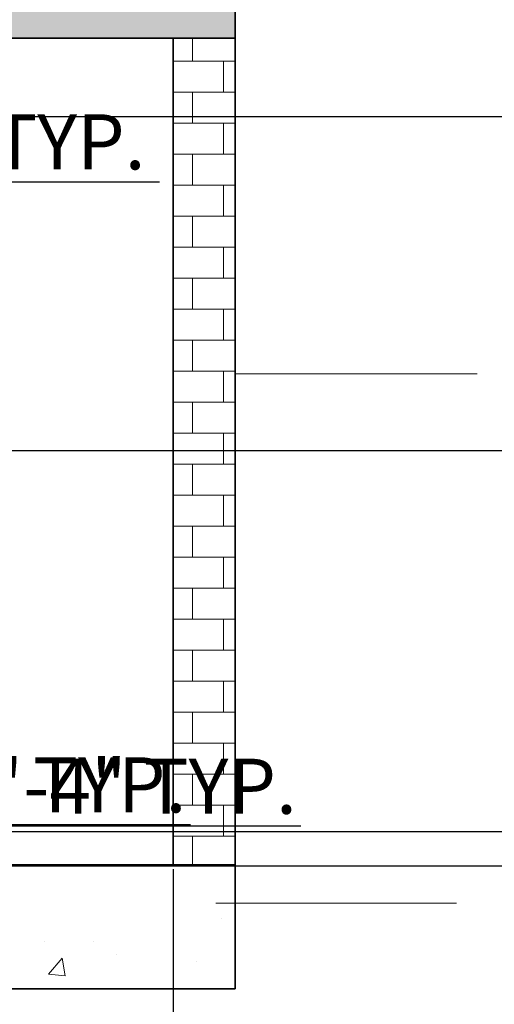
# Model space of a CAD drawing. Units: inches. Extents: x 2257 to 3678, y 834 to 1975.
# Tile 14 of 16: x 3471 to 3540, y 1677 to 1820. Entities that reach past the tile are written whole.
import ezdxf

# ---------------------------------------------------------------- set-up
doc = ezdxf.new("R2010")
doc.units = ezdxf.units.IN
for name, color, linetype, lineweight in [('A-ANNO-DIMS', 2, 'Continuous', 18), ('A-ANNO-TEXT', 7, 'Continuous', 18), ('A-SECT', 7, 'Continuous', 35), ('A-SECT-BRCK-PATT', 252, 'Continuous', 13), ('A-SECT-CONC-PATT', 252, 'Continuous', 13)]:
    doc.layers.add(name, color=color, linetype=linetype, lineweight=lineweight)
doc.styles.get("Standard").update_dxf_attribs({"font": 'arial.ttf'})
doc.dimstyles.new('ISO-25', dxfattribs={"dimtxt": 8, "dimasz": 2.5, "dimexe": 1.25, "dimexo": 0.625, "dimtad": 1, "dimdec": 0, "dimlunit": 3, "dimtxsty": 'Standard', "dimcen": 2.5, "dimadec": 0, "dimazin": 0, "dimtfac": 1, "dimtdec": 0, "dimtmove": 0, "dimatfit": 3, "dimfxl": 1, "dimarcsym": 0})

# ---------------------------------------------------------------- blocks, each defined once
blk = doc.blocks.new('*D84')
at = {"layer": 'A-ANNO-DIMS', "color": 0, "lineweight": -2, "transparency": 16777216}
for p, q in [((3377.06, 1793.76), (3377.06, 1797.23)), ((3396.05, 1793.76), (3396.05, 1797.23)), ((3379.56, 1795.98), (3393.55, 1795.98)), ((3396.05, 1795.98), (3491.69, 1795.98))]:
    blk.add_line(p, q, dxfattribs=at)
at = {"layer": 'A-ANNO-DIMS', "color": 0, "transparency": 16777216}
for points in [[(3379.56, 1796.4), (3379.56, 1795.56), (3377.06, 1795.98)], [(3393.55, 1796.4), (3393.55, 1795.56), (3396.05, 1795.98)]]:
    blk.add_solid(points, dxfattribs=at)
at = {"layer": 'Defpoints', "color": 0, "transparency": 16777216}
for p in [(3396.05, 1795.98), (3377.06, 1793.13), (3396.05, 1793.13)]:
    blk.add_point(p, dxfattribs=at)
at = {"layer": 'A-ANNO-DIMS', "color": 0, "transparency": 16777216, "insert": (3445.12, 1800.74), "char_height": 8, "attachment_point": 5}
blk.add_mtext('LINENS 1\'-7" TYP.', dxfattribs=at)
blk = doc.blocks.new('*D90')
at = {"layer": 'A-ANNO-DIMS', "color": 0, "lineweight": -2, "transparency": 16777216}
for p, q in [((3463.51, 1750.62), (3463.51, 1883.51)), ((3457.86, 1750.62), (3464.76, 1750.62)), ((3463.51, 1711.27), (3463.51, 1748.12)), ((3457.86, 1708.77), (3464.76, 1708.77))]:
    blk.add_line(p, q, dxfattribs=at)
at = {"layer": 'A-ANNO-DIMS', "color": 0, "transparency": 16777216}
for points in [[(3463.09, 1748.12), (3463.92, 1748.12), (3463.51, 1750.62)], [(3463.09, 1711.27), (3463.92, 1711.27), (3463.51, 1708.77)]]:
    blk.add_solid(points, dxfattribs=at)
at = {"layer": 'Defpoints', "color": 0, "transparency": 16777216}
for p in [(3457.23, 1750.62), (3463.51, 1750.62), (3457.23, 1708.77)]:
    blk.add_point(p, dxfattribs=at)
at = {"layer": 'A-ANNO-DIMS', "color": 0, "transparency": 16777216, "insert": (3458.74, 1818.32), "char_height": 8, "attachment_point": 5, "rotation": 90}
blk.add_mtext('LONG JACKET 3\'-6" TYP.', dxfattribs=at)
blk = doc.blocks.new('*D91')
at = {"layer": 'A-ANNO-DIMS', "color": 0, "lineweight": -2, "transparency": 16777216}
for p, q in [((3453, 1708.14), (3453, 1701.24)), ((3457.23, 1708.14), (3457.23, 1701.24)), ((3450.5, 1702.49), (3448, 1702.49)), ((3453, 1702.49), (3457.23, 1702.49)), ((3459.73, 1702.49), (3512.24, 1702.49))]:
    blk.add_line(p, q, dxfattribs=at)
at = {"layer": 'A-ANNO-DIMS', "color": 0, "transparency": 16777216}
for points in [[(3450.5, 1702.91), (3450.5, 1702.08), (3453, 1702.49)], [(3459.73, 1702.91), (3459.73, 1702.08), (3457.23, 1702.49)]]:
    blk.add_solid(points, dxfattribs=at)
at = {"layer": 'Defpoints', "color": 0, "transparency": 16777216}
for p in [(3453, 1708.77), (3457.23, 1708.77), (3457.23, 1702.49)]:
    blk.add_point(p, dxfattribs=at)
at = {"layer": 'A-ANNO-DIMS', "color": 0, "transparency": 16777216, "insert": (3487.24, 1707.2), "char_height": 8, "attachment_point": 5}
blk.add_mtext('0\'-4" TYP.', dxfattribs=at)
blk = doc.blocks.new('*D93')
at = {"layer": 'A-ANNO-DIMS', "color": 0, "lineweight": -2, "transparency": 16777216}
for p, q in [((3435.17, 1708.31), (3435.17, 1701.44)), ((3441.18, 1708.31), (3441.18, 1701.44)), ((3432.67, 1702.69), (3430.17, 1702.69)), ((3435.17, 1702.69), (3441.18, 1702.69)), ((3443.68, 1702.69), (3496.2, 1702.69))]:
    blk.add_line(p, q, dxfattribs=at)
at = {"layer": 'A-ANNO-DIMS', "color": 0, "transparency": 16777216}
for points in [[(3432.67, 1703.11), (3432.67, 1702.27), (3435.17, 1702.69)], [(3443.68, 1703.11), (3443.68, 1702.27), (3441.18, 1702.69)]]:
    blk.add_solid(points, dxfattribs=at)
at = {"layer": 'Defpoints', "color": 0, "transparency": 16777216}
for p in [(3435.17, 1708.94), (3441.18, 1708.94), (3441.18, 1702.69)]:
    blk.add_point(p, dxfattribs=at)
at = {"layer": 'A-ANNO-DIMS', "color": 0, "transparency": 16777216, "insert": (3471.19, 1707.4), "char_height": 8, "attachment_point": 5}
blk.add_mtext('0\'-6" TYP.', dxfattribs=at)
blk = doc.blocks.new('*D137')
at = {"layer": 'A-ANNO-DIMS', "color": 0, "lineweight": -2, "transparency": 16777216}
for p, q in [((3337.7, 1696.22), (3337.7, 1600.44)), ((3493.7, 1696.22), (3493.7, 1600.44)), ((3340.2, 1601.69), (3491.2, 1601.69))]:
    blk.add_line(p, q, dxfattribs=at)
at = {"layer": 'A-ANNO-DIMS', "color": 0, "transparency": 16777216}
for points in [[(3340.2, 1602.1), (3340.2, 1601.27), (3337.7, 1601.69)], [(3491.2, 1602.1), (3491.2, 1601.27), (3493.7, 1601.69)]]:
    blk.add_solid(points, dxfattribs=at)
at = {"layer": 'Defpoints', "color": 0, "transparency": 16777216}
for p in [(3337.7, 1696.84), (3493.7, 1696.84), (3493.7, 1601.69)]:
    blk.add_point(p, dxfattribs=at)
at = {"layer": 'A-ANNO-DIMS', "color": 0, "transparency": 16777216, "insert": (3415.7, 1606.4), "char_height": 8, "attachment_point": 5}
blk.add_mtext('13\'-0"', dxfattribs=at)
blk = doc.blocks.new('*D139')
at = {"layer": 'A-ANNO-DIMS', "color": 0, "lineweight": -2, "transparency": 16777216}
for p, q in [((3463.29, 1805.46), (3573.28, 1805.46)), ((3572.03, 1699.2), (3572.03, 1802.96)), ((3463.29, 1696.7), (3573.28, 1696.7))]:
    blk.add_line(p, q, dxfattribs=at)
at = {"layer": 'A-ANNO-DIMS', "color": 0, "transparency": 16777216}
for points in [[(3571.61, 1802.96), (3572.45, 1802.96), (3572.03, 1805.46)], [(3571.61, 1699.2), (3572.45, 1699.2), (3572.03, 1696.7)]]:
    blk.add_solid(points, dxfattribs=at)
at = {"layer": 'Defpoints', "color": 0, "transparency": 16777216}
for p in [(3462.66, 1805.46), (3572.03, 1805.46), (3462.66, 1696.7)]:
    blk.add_point(p, dxfattribs=at)
at = {"layer": 'A-ANNO-DIMS', "color": 0, "transparency": 16777216, "insert": (3567.32, 1751.08), "char_height": 8, "attachment_point": 5, "rotation": 90}
blk.add_mtext('9\'-1"', dxfattribs=at)
blk = doc.blocks.new('*D147')
at = {"layer": 'A-ANNO-DIMS', "color": 0, "lineweight": -2, "transparency": 16777216}
for p, q in [((3460.57, 1756.97), (3573.28, 1756.97)), ((3572.03, 1704.19), (3572.03, 1754.47)), ((3460.57, 1701.69), (3573.28, 1701.69))]:
    blk.add_line(p, q, dxfattribs=at)
at = {"layer": 'A-ANNO-DIMS', "color": 0, "transparency": 16777216}
for points in [[(3571.61, 1754.47), (3572.45, 1754.47), (3572.03, 1756.97)], [(3571.61, 1704.19), (3572.45, 1704.19), (3572.03, 1701.69)]]:
    blk.add_solid(points, dxfattribs=at)
at = {"layer": 'Defpoints', "color": 0, "transparency": 16777216}
for p in [(3459.94, 1756.97), (3572.03, 1756.97), (3459.94, 1701.69)]:
    blk.add_point(p, dxfattribs=at)
at = {"layer": 'A-ANNO-DIMS', "color": 0, "transparency": 16777216, "insert": (3567.27, 1729.33), "char_height": 8, "attachment_point": 5, "rotation": 90}
blk.add_mtext('4\'-7 1/2"', dxfattribs=at)

msp = doc.modelspace()

# ---------------------------------------------------------------- hatches: boundary and pattern name
at = {"layer": 'A-SECT-BRCK-PATT'}
h = msp.add_hatch(dxfattribs=at)
h.set_pattern_fill('BRICK', color=256, scale=0.708661, style=0)
h.paths.add_polyline_path([(3493.7, 1696.84), (3502.7, 1696.84), (3502.7, 1816.84), (3493.7, 1816.84)])
at = {"layer": 'A-SECT-CONC-PATT'}
h = msp.add_hatch(dxfattribs=at)
h.set_pattern_fill('AR-CONC', color=256, scale=0.035, style=0)
h.paths.add_polyline_path([(3004.7, 1816.84), (3502.7, 1816.84), (3502.7, 1822.84), (3004.7, 1822.84)])
h = msp.add_hatch(dxfattribs=at)
h.set_pattern_fill('AR-CONC', color=256, scale=0.16, style=0)
h.paths.add_polyline_path([(3004.7, 1678.84), (3502.7, 1678.84), (3502.7, 1696.84), (3004.7, 1696.84)])

# ---------------------------------------------------------------- linework, layer by layer
at = {"layer": 'A-ANNO-TEXT'}
for p, q in [((3502.7, 1768.09), (3537.81, 1768.09)), ((3499.86, 1691.27), (3534.81, 1691.27))]:
    msp.add_line(p, q, dxfattribs=at)
at = {"layer": 'A-SECT'}
for p, q in [((3502.7, 1864.84), (3502.7, 1678.84)), ((3502.7, 1816.84), (3196.31, 1816.84)), ((3493.7, 1816.84), (3493.7, 1696.84)), ((3502.7, 1696.84), (3004.7, 1696.84)), ((3502.7, 1678.84), (3004.7, 1678.84))]:
    msp.add_line(p, q, dxfattribs=at)

# ---------------------------------------------------------------- dimensions: what is measured, and where the dimension line sits
at = {"layer": 'A-ANNO-DIMS'}
dim = msp.add_linear_dim(base=(3463.5083, 1750.6208), p1=(3457.2306, 1708.7697), p2=(3457.2306, 1750.6208), angle=90, text='LONG JACKET <> TYP.', dimstyle='ISO-25', override={"dimdec": 1, "dimlfac": 1, "dimrnd": 0, "dimzin": 1, "dimdsep": 46, "dimlunit": 4, "dimfrac": 2}, dxfattribs=at)
dim.commit()
dim.dimension.update_dxf_attribs({"geometry": '*D90', "text_midpoint": (3458.7414, 1818.3161)})
for base, p1, p2, text, picture, middle in [((3396.05, 1795.98), (3377.06, 1793.13), (3396.05, 1793.13), 'LINENS <> TYP.', '*D84', (3445.12, 1800.74)), ((3441.18, 1702.69), (3435.17, 1708.94), (3441.18, 1708.94), '<> TYP.', '*D93', (3471.19, 1707.4)), ((3457.23, 1702.49), (3453, 1708.77), (3457.23, 1708.77), '<> TYP.', '*D91', (3487.24, 1707.2))]:
    dim = msp.add_linear_dim(base=base, p1=p1, p2=p2, text=text, dimstyle='ISO-25', override={"dimdec": 1, "dimlfac": 1, "dimrnd": 0, "dimzin": 1, "dimdsep": 46, "dimlunit": 4, "dimfrac": 2}, dxfattribs=at)
    dim.commit()
    dim.dimension.update_dxf_attribs({"geometry": picture, "text_midpoint": middle})
for base, p1, p2, picture, middle in [((3572.03, 1805.46), (3462.66, 1696.7), (3462.66, 1805.46), '*D139', (3567.32, 1751.08)), ((3572.03, 1756.97), (3459.94, 1701.69), (3459.94, 1756.97), '*D147', (3567.27, 1729.33))]:
    dim = msp.add_linear_dim(base=base, p1=p1, p2=p2, angle=90, dimstyle='ISO-25', override={"dimdec": 1, "dimlfac": 1, "dimrnd": 0, "dimzin": 1, "dimdsep": 46, "dimlunit": 4, "dimfrac": 2}, dxfattribs=at)
    dim.commit()
    dim.dimension.update_dxf_attribs({"geometry": picture, "text_midpoint": middle})
dim = msp.add_linear_dim(base=(3493.7, 1601.69), p1=(3337.7, 1696.84), p2=(3493.7, 1696.84), dimstyle='ISO-25', override={"dimdec": 1, "dimlfac": 1, "dimrnd": 0, "dimzin": 1, "dimdsep": 46, "dimlunit": 4, "dimfrac": 2}, dxfattribs=at)
dim.commit()
dim.dimension.update_dxf_attribs({"geometry": '*D137', "text_midpoint": (3415.7, 1606.4)})

doc.saveas('drawing.dxf')
